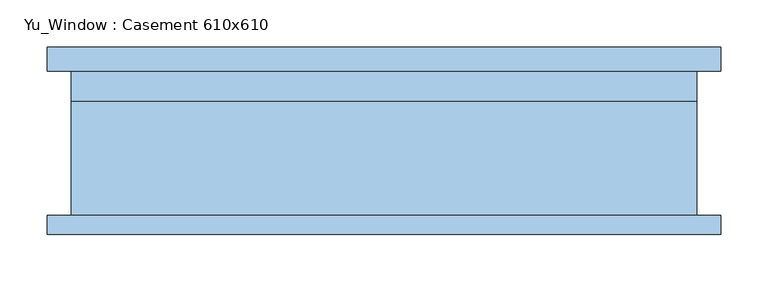
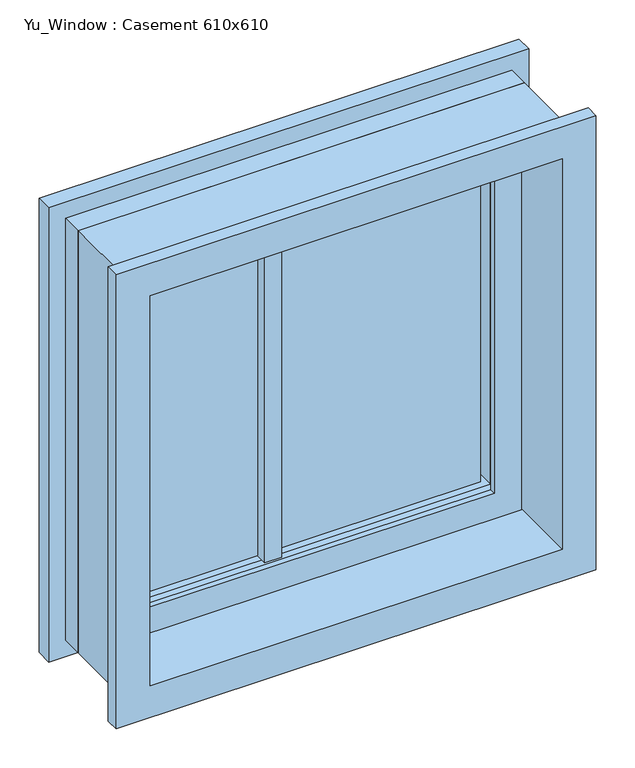
"""IFC4 building model written with IfcOpenShell, lengths in millimetres: window geometry, Yu_Window : Casement 610x610."""

from ifc_helpers import new_model, si_unit, frame, origin, place, context, project, spatial, polyline, outline, extrude, faceted_brep, source, transform, mapped, element, save


def yu_window_casement_610x610_b7484dfd(model_context):
    return source(origin(), model_context, "Body", "SolidModel", [
        faceted_brep([(279.8, 23.8, 1184.6), (279.8, 43.8, 1184.6), (279.8, 43.8, 625.0), (279.8, 23.8, 625.0), (329.8, 43.8, 1234.6), (329.8, 43.8, 575.0), (-329.8, 43.8, 575.0), (-329.8, 43.8, 1234.6), (-279.8, 43.8, 1184.6), (-279.8, 43.8, 625.0), (-279.8, 23.8, 625.0), (-304.8, 23.8, 1209.6), (-304.8, 23.8, 600.0), (304.8, 23.8, 600.0), (304.8, 23.8, 1209.6), (-279.8, 23.8, 1184.6), (304.8, -96.2, 1209.6), (304.8, -96.2, 600.0), (-304.8, -96.2, 600.0), (-354.8, -96.2, 1259.6), (-354.8, -96.2, 550.0), (354.8, -96.2, 550.0), (354.8, -96.2, 1259.6), (-304.8, -96.2, 1209.6), (354.8, -76.2, 1259.6), (354.8, -76.2, 550.0), (-354.8, -76.2, 550.0), (-354.8, -76.2, 1259.6), (-329.8, -76.2, 1234.6), (-329.8, -76.2, 575.0), (329.8, -76.2, 575.0), (329.8, -76.2, 1234.6)], [[[0, 1, 2, 3]], [[4, 5, 6, 7], [8, 9, 2, 1]], [[3, 2, 9, 10]], [[11, 12, 13, 14], [0, 3, 10, 15]], [[16, 14, 13, 17]], [[17, 13, 12, 18]], [[19, 20, 21, 22], [16, 17, 18, 23]], [[24, 22, 21, 25]], [[25, 21, 20, 26]], [[24, 25, 26, 27], [28, 29, 30, 31]], [[4, 31, 30, 5]], [[5, 30, 29, 6]], [[10, 9, 8, 15]], [[18, 12, 11, 23]], [[26, 20, 19, 27]], [[6, 29, 28, 7]], [[15, 8, 1, 0]], [[23, 11, 14, 16]], [[27, 19, 22, 24]], [[7, 28, 31, 4]]]),
        faceted_brep([(-279.8, 68.8, 1184.6), (-279.8, 43.8, 1184.6), (-279.8, 43.8, 625.0), (-279.8, 68.8, 625.0), (-329.8, 43.8, 1234.6), (-329.8, 43.8, 575.0), (329.8, 43.8, 575.0), (329.8, 43.8, 1234.6), (279.8, 43.8, 1184.6), (279.8, 43.8, 625.0), (279.8, 68.8, 625.0), (304.8, 68.8, 1209.6), (304.8, 68.8, 600.0), (-304.8, 68.8, 600.0), (-304.8, 68.8, 1209.6), (279.8, 68.8, 1184.6), (-304.8, 101.2, 1209.6), (-304.8, 101.2, 600.0), (304.8, 101.2, 600.0), (354.8, 101.2, 1259.6), (354.8, 101.2, 550.0), (-354.8, 101.2, 550.0), (-354.8, 101.2, 1259.6), (304.8, 101.2, 1209.6), (-354.8, 76.2, 1259.6), (-354.8, 76.2, 550.0), (354.8, 76.2, 550.0), (354.8, 76.2, 1259.6), (329.8, 76.2, 1234.6), (329.8, 76.2, 575.0), (-329.8, 76.2, 575.0), (-329.8, 76.2, 1234.6)], [[[0, 1, 2, 3]], [[4, 5, 6, 7], [8, 9, 2, 1]], [[3, 2, 9, 10]], [[11, 12, 13, 14], [0, 3, 10, 15]], [[16, 14, 13, 17]], [[17, 13, 12, 18]], [[19, 20, 21, 22], [16, 17, 18, 23]], [[24, 22, 21, 25]], [[25, 21, 20, 26]], [[24, 25, 26, 27], [28, 29, 30, 31]], [[4, 31, 30, 5]], [[5, 30, 29, 6]], [[10, 9, 8, 15]], [[18, 12, 11, 23]], [[26, 20, 19, 27]], [[6, 29, 28, 7]], [[15, 8, 1, 0]], [[23, 11, 14, 16]], [[27, 19, 22, 24]], [[7, 28, 31, 4]]]),
        extrude(outline(polyline([(605.0, 299.8), (1204.6, 299.8), (1204.6, -299.8), (605.0, -299.8), (605.0, 299.8)]), holes=[polyline([(645.0, -259.8), (1164.6, -259.8), (1164.6, 259.8), (645.0, 259.8), (645.0, -259.8)])]), frame((0.0, 0.0, 0.0), z_axis=(0.0, 1.0, 0.0), x_axis=(0.0, 0.0, 1.0)), (0.0, 0.0, 1.0), 8.8),
        extrude(outline(polyline([(605.0, 299.8), (1204.6, 299.8), (1204.6, -299.8), (605.0, -299.8), (605.0, 299.8)]), holes=[polyline([(655.0, -249.8), (1154.6, -249.8), (1154.6, 249.8), (655.0, 249.8), (655.0, -249.8)])]), frame((0.0, 68.8, 0.0), z_axis=(0.0, 1.0, 0.0), x_axis=(0.0, 0.0, 1.0)), (0.0, 0.0, 1.0), 15.0),
        extrude(outline(polyline([(-249.8, 22.0), (249.8, 22.0), (249.8, 18.0), (-249.8, 18.0), (-249.8, 22.0)])), frame((0.0, 0.0, 655.0), z_axis=(0.0, 0.0, 1.0), x_axis=(1.0, 0.0, 0.0)), (0.0, 0.0, 1.0), 499.6),
        extrude(outline(polyline([(-54.8, 68.8), (-54.8, 0.0), (-79.8, 0.0), (-79.8, 68.8), (-54.8, 68.8)])), frame((0.0, 0.0, 655.0), z_axis=(0.0, 0.0, 1.0), x_axis=(1.0, 0.0, 0.0)), (0.0, 0.0, 1.0), 549.6),
        extrude(outline(polyline([(-259.8, 18.0), (-259.8, 22.0), (259.8, 22.0), (259.8, 18.0), (-259.8, 18.0)])), frame((0.0, 0.0, 1184.6), z_axis=(0.0, 0.0, 1.0), x_axis=(1.0, 0.0, 0.0)), (0.0, 0.0, 1.0), 25.0),
    ])


if __name__ == "__main__":
    model = new_model("IFC4")
    model_context = context("Model", 3, world=origin())
    ifc_project = project(units=[si_unit("LENGTHUNIT", "METRE", prefix="MILLI")], contexts=[model_context])
    site = spatial("IfcSite", under=ifc_project)
    building = spatial("IfcBuilding", under=site)
    placement = place(None, origin())
    yu_window_casement_610x610_shape = yu_window_casement_610x610_b7484dfd(model_context)
    element("IfcWindow", 1, ObjectType="Yu_Window : Casement 610x610", at=placement, inside=building, context=model_context, shape_type="MappedRepresentation", body=[
        mapped(yu_window_casement_610x610_shape, transform((0.0, 0.0, 0.0), x_axis=(1.0, 0.0, 0.0), y_axis=(0.0, 1.0, 0.0), z_axis=(0.0, 0.0, 1.0))),
    ])
    save(model, "model.ifc")

# Revit data of these elements
# Type "Yu_Window : Casement 610x610"
#   Type Mark = "25"
#   Analytic Construction = "<None>"
#   mullion 2 = 0' - 0"
#   Window panel size 1 = 0' - 8.85827"
#   Offset = 0' - 0.98425"
#   Height = 2' - 0"
#   Default Sill Height = 1' - 11.62205"
#   Width = 2' - 0"
#   Define Thermal Properties by = 1
#   Interior material = none
#   Exterior material = none
#   Wall Closure = (empty or 0)
# Element 1 (IfcWindow, "Yu_Window : Casement 610x610")
#   Materials on its faces: "Glass"
# Materials
#   "Glass": class "Glass", colour RGB 0 128 192, transparency 0.75, Description = "Soda Lime Glass", Cost = 0
